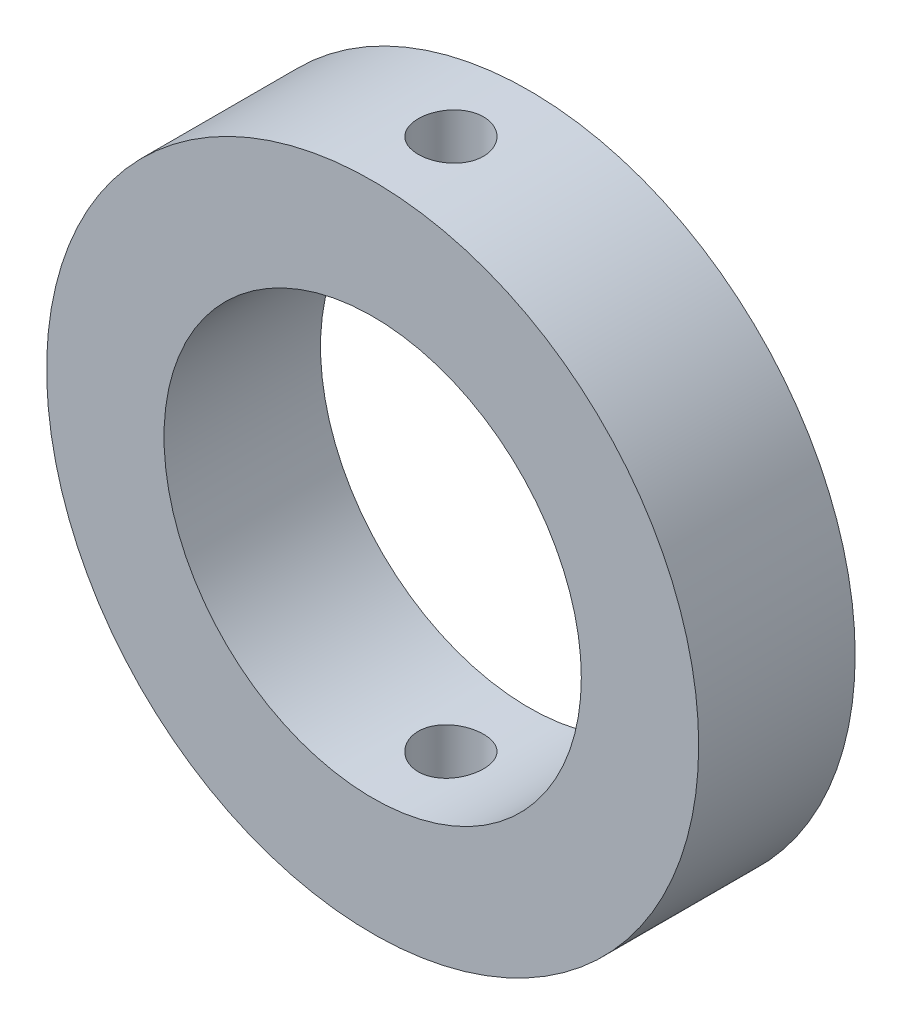
ISO-10303-21;
HEADER;
FILE_DESCRIPTION(('STEP AP214'),'2;1');
FILE_NAME('part.step','',(''),(''),'','','');
FILE_SCHEMA(('AUTOMOTIVE_DESIGN { 1 0 10303 214 1 1 1 1 }'));
ENDSEC;
DATA;
#1=APPLICATION_CONTEXT('core data for automotive mechanical design processes');
#2=APPLICATION_PROTOCOL_DEFINITION('international standard','automotive_design',2000,#1);
#3=PRODUCT_CONTEXT('',#1,'mechanical');
#4=PRODUCT('Part','Part','',(#3));
#5=PRODUCT_RELATED_PRODUCT_CATEGORY('part','',(#4));
#6=PRODUCT_DEFINITION_FORMATION('','',#4);
#7=PRODUCT_DEFINITION_CONTEXT('part definition',#1,'design');
#8=PRODUCT_DEFINITION('design','',#6,#7);
#9=PRODUCT_DEFINITION_SHAPE('','',#8);
#10=(LENGTH_UNIT() NAMED_UNIT(*) SI_UNIT(.MILLI.,.METRE.));
#11=(NAMED_UNIT(*) PLANE_ANGLE_UNIT() SI_UNIT($,.RADIAN.));
#12=(NAMED_UNIT(*) SI_UNIT($,.STERADIAN.) SOLID_ANGLE_UNIT());
#13=UNCERTAINTY_MEASURE_WITH_UNIT(LENGTH_MEASURE(1.E-05),#10,'distance_accuracy_value','');
#14=(GEOMETRIC_REPRESENTATION_CONTEXT(3) GLOBAL_UNCERTAINTY_ASSIGNED_CONTEXT((#13)) GLOBAL_UNIT_ASSIGNED_CONTEXT((#10,
#11,#12)) REPRESENTATION_CONTEXT('',''));
#15=CARTESIAN_POINT('',(0.,0.,0.));
#16=DIRECTION('',(0.,0.,1.));
#17=DIRECTION('',(1.,0.,0.));
#18=AXIS2_PLACEMENT_3D('',#15,#16,#17);
#19=CARTESIAN_POINT('',(0.,0.,12.));
#20=DIRECTION('',(0.,0.,1.));
#21=DIRECTION('',(1.,0.,0.));
#22=AXIS2_PLACEMENT_3D('',#19,#20,#21);
#23=PLANE('',#22);
#24=CARTESIAN_POINT('',(0.,0.,12.));
#25=DIRECTION('',(0.,0.,1.));
#26=DIRECTION('',(1.,0.,0.));
#27=AXIS2_PLACEMENT_3D('',#24,#25,#26);
#28=CIRCLE('',#27,25.);
#29=CARTESIAN_POINT('',(25.,0.,12.));
#30=VERTEX_POINT('',#29);
#31=EDGE_CURVE('E10',#30,#30,#28,.T.);
#32=ORIENTED_EDGE('',*,*,#31,.T.);
#33=EDGE_LOOP('',(#32));
#34=FACE_BOUND('',#33,.T.);
#35=CARTESIAN_POINT('',(0.,0.,12.));
#36=DIRECTION('',(0.,0.,1.));
#37=DIRECTION('',(1.,0.,0.));
#38=AXIS2_PLACEMENT_3D('',#35,#36,#37);
#39=CIRCLE('',#38,16.);
#40=CARTESIAN_POINT('',(16.,0.,12.));
#41=VERTEX_POINT('',#40);
#42=EDGE_CURVE('E57',#41,#41,#39,.T.);
#43=ORIENTED_EDGE('',*,*,#42,.F.);
#44=EDGE_LOOP('',(#43));
#45=FACE_BOUND('',#44,.T.);
#46=ADVANCED_FACE('F40',(#34,#45),#23,.T.);
#47=CARTESIAN_POINT('',(0.,0.,0.));
#48=DIRECTION('',(0.,0.,1.));
#49=DIRECTION('',(1.,0.,0.));
#50=AXIS2_PLACEMENT_3D('',#47,#48,#49);
#51=PLANE('',#50);
#52=CARTESIAN_POINT('',(0.,0.,0.));
#53=DIRECTION('',(0.,0.,1.));
#54=DIRECTION('',(1.,0.,0.));
#55=AXIS2_PLACEMENT_3D('',#52,#53,#54);
#56=CIRCLE('',#55,25.);
#57=CARTESIAN_POINT('',(25.,0.,0.));
#58=VERTEX_POINT('',#57);
#59=EDGE_CURVE('E51',#58,#58,#56,.T.);
#60=ORIENTED_EDGE('',*,*,#59,.F.);
#61=EDGE_LOOP('',(#60));
#62=FACE_BOUND('',#61,.T.);
#63=CARTESIAN_POINT('',(0.,0.,0.));
#64=DIRECTION('',(0.,0.,1.));
#65=DIRECTION('',(1.,0.,0.));
#66=AXIS2_PLACEMENT_3D('',#63,#64,#65);
#67=CIRCLE('',#66,16.);
#68=CARTESIAN_POINT('',(16.,0.,0.));
#69=VERTEX_POINT('',#68);
#70=EDGE_CURVE('E56',#69,#69,#67,.T.);
#71=ORIENTED_EDGE('',*,*,#70,.T.);
#72=EDGE_LOOP('',(#71));
#73=FACE_BOUND('',#72,.T.);
#74=ADVANCED_FACE('F92',(#62,#73),#51,.F.);
#75=CARTESIAN_POINT('',(0.,0.,12.));
#76=DIRECTION('',(0.,0.,-1.));
#77=DIRECTION('',(-1.,0.,0.));
#78=AXIS2_PLACEMENT_3D('',#75,#76,#77);
#79=CYLINDRICAL_SURFACE('',#78,25.);
#80=CARTESIAN_POINT('',(0.,-25.,8.5));
#81=CARTESIAN_POINT('',(0.140050884478893,-24.9999983880192,8.49999393524905));
#82=CARTESIAN_POINT('',(0.280194362919433,-24.9988106399051,8.48819182775889));
#83=CARTESIAN_POINT('',(0.556595996242092,-24.9941866898684,8.44128907427393));
#84=CARTESIAN_POINT('',(0.69284969792207,-24.9907480108506,8.40616275993853));
#85=CARTESIAN_POINT('',(0.957429188633536,-24.9820103640768,8.31364439850542));
#86=CARTESIAN_POINT('',(1.08575971153727,-24.9767125200177,8.25626579870382));
#87=CARTESIAN_POINT('',(1.33094040240102,-24.9648489348577,8.12089773017089));
#88=CARTESIAN_POINT('',(1.44779284694769,-24.9582834459533,8.04291235999965));
#89=CARTESIAN_POINT('',(1.66714887668521,-24.9445936085331,7.86824325584432));
#90=CARTESIAN_POINT('',(1.76960536208723,-24.9374675393466,7.77150050149492));
#91=CARTESIAN_POINT('',(1.95685630357746,-24.9234739226566,7.56218866434242));
#92=CARTESIAN_POINT('',(2.04164994270663,-24.9166063871229,7.44961884989403));
#93=CARTESIAN_POINT('',(2.19133492610904,-24.9038897888196,7.21155367079095));
#94=CARTESIAN_POINT('',(2.2561836636372,-24.8980429177726,7.08603138976285));
#95=CARTESIAN_POINT('',(2.3638659618569,-24.8880509386631,6.82581103523755));
#96=CARTESIAN_POINT('',(2.40670006647823,-24.8839057885556,6.69111318854013));
#97=CARTESIAN_POINT('',(2.46899760400473,-24.8778021018244,6.41684549783498));
#98=CARTESIAN_POINT('',(2.48853913250949,-24.8758362599524,6.27729355786948));
#99=CARTESIAN_POINT('',(2.5039382128384,-24.8742910765131,5.99687784151055));
#100=CARTESIAN_POINT('',(2.499796387177,-24.8747116722186,5.85601409969485));
#101=CARTESIAN_POINT('',(2.4680107006317,-24.8778851724734,5.5775117257667));
#102=CARTESIAN_POINT('',(2.44045211031138,-24.8806296147663,5.43986325167826));
#103=CARTESIAN_POINT('',(2.36274786037647,-24.8881283571855,5.17115509199726));
#104=CARTESIAN_POINT('',(2.31260189563937,-24.8928826844623,5.04009549543742));
#105=CARTESIAN_POINT('',(2.19105223470377,-24.9038752363018,4.78801603175278));
#106=CARTESIAN_POINT('',(2.11961070679995,-24.9101160977039,4.66701452627671));
#107=CARTESIAN_POINT('',(1.95752506838307,-24.923376293322,4.43868696272029));
#108=CARTESIAN_POINT('',(1.86688039584126,-24.9303956503196,4.33136130504559));
#109=CARTESIAN_POINT('',(1.66848528103017,-24.9444596328247,4.13293651502743));
#110=CARTESIAN_POINT('',(1.56066119712841,-24.9515042333249,4.04191099529799));
#111=CARTESIAN_POINT('',(1.33122370434278,-24.964795726963,3.87924091772403));
#112=CARTESIAN_POINT('',(1.209610279999,-24.9710426192064,3.80759638160881));
#113=CARTESIAN_POINT('',(0.955995264230911,-24.9820368916774,3.68572494922437));
#114=CARTESIAN_POINT('',(0.823991865974758,-24.9867840103692,3.63550178795485));
#115=CARTESIAN_POINT('',(0.55336804332483,-24.9942411860352,3.55795270822062));
#116=CARTESIAN_POINT('',(0.414747816941501,-24.9969513039266,3.53062610502344));
#117=CARTESIAN_POINT('',(0.135462747729759,-25.0000212917078,3.49973923066309));
#118=CARTESIAN_POINT('',(-0.00519075526372992,-25.0003912066934,3.49607737936875));
#119=CARTESIAN_POINT('',(-0.285109483289249,-24.9987660439199,3.51235715762191));
#120=CARTESIAN_POINT('',(-0.424374727051175,-24.9967709981117,3.5322984682882));
#121=CARTESIAN_POINT('',(-0.697270517086687,-24.9906465384799,3.59513423855394));
#122=CARTESIAN_POINT('',(-0.830912122430048,-24.986521547951,3.63798113619503));
#123=CARTESIAN_POINT('',(-1.08911080345945,-24.9765999715152,3.74536293509318));
#124=CARTESIAN_POINT('',(-1.21366767539279,-24.9708033481313,3.80989832259849));
#125=CARTESIAN_POINT('',(-1.45062045043036,-24.9581618832606,3.95907709665978));
#126=CARTESIAN_POINT('',(-1.56297414937229,-24.951313590086,4.04378722231454));
#127=CARTESIAN_POINT('',(-1.7719040582797,-24.937348321738,4.23081516935232));
#128=CARTESIAN_POINT('',(-1.86847987212294,-24.9302313398243,4.33313343267579));
#129=CARTESIAN_POINT('',(-2.04346527471786,-24.9165006035189,4.5529164366475));
#130=CARTESIAN_POINT('',(-2.12180819669886,-24.9098887534744,4.67043439135655));
#131=CARTESIAN_POINT('',(-2.25764564685957,-24.8979458115222,4.91701840036671));
#132=CARTESIAN_POINT('',(-2.31514046013471,-24.8926147021009,5.04608429672099));
#133=CARTESIAN_POINT('',(-2.40753802171119,-24.8838486908512,5.31187184866449));
#134=CARTESIAN_POINT('',(-2.44248043702965,-24.8804104612447,5.4485796002278));
#135=CARTESIAN_POINT('',(-2.48891001782366,-24.8758091320719,5.72595799490193));
#136=CARTESIAN_POINT('',(-2.50039785599879,-24.8746459672547,5.86662852423918));
#137=CARTESIAN_POINT('',(-2.49958284617814,-24.8747278276891,6.14727672089176));
#138=CARTESIAN_POINT('',(-2.48738472398278,-24.8759622521752,6.28725470720704));
#139=CARTESIAN_POINT('',(-2.43976363240913,-24.8806775972386,6.56316229292072));
#140=CARTESIAN_POINT('',(-2.4043406369054,-24.884158520343,6.69909188776495));
#141=CARTESIAN_POINT('',(-2.31130421574376,-24.8929717065797,6.96304337261964));
#142=CARTESIAN_POINT('',(-2.25369386085229,-24.898303713509,7.09106635407431));
#143=CARTESIAN_POINT('',(-2.11792888727761,-24.910218795984,7.33564222917759));
#144=CARTESIAN_POINT('',(-2.03977438363854,-24.9168018645238,7.45219518705157));
#145=CARTESIAN_POINT('',(-1.86474639071333,-24.9305121802424,7.67105918617984));
#146=CARTESIAN_POINT('',(-1.76779487222567,-24.9376416181688,7.77330769091772));
#147=CARTESIAN_POINT('',(-1.55807924806277,-24.9516213682196,7.96013058174914));
#148=CARTESIAN_POINT('',(-1.44531136027064,-24.9584716130744,8.04470072839292));
#149=CARTESIAN_POINT('',(-1.20685358540322,-24.971139051729,8.19393363463655));
#150=CARTESIAN_POINT('',(-1.08113187336691,-24.9769536006703,8.25854572736296));
#151=CARTESIAN_POINT('',(-0.820645697751378,-24.9868657312474,8.36565605705967));
#152=CARTESIAN_POINT('',(-0.685891624564024,-24.9909652477413,8.40817922738387));
#153=CARTESIAN_POINT('',(-0.458645653514261,-24.9959553443433,8.45930154271201));
#154=CARTESIAN_POINT('',(-0.367606382111272,-24.9974650172958,8.47454261074839));
#155=CARTESIAN_POINT('',(-0.184391452043282,-24.9994878737697,8.4948938151544));
#156=CARTESIAN_POINT('',(-0.0922157980663944,-25.0000010614006,8.50000399330465));
#157=CARTESIAN_POINT('',(0.,-25.,8.5));
#158=B_SPLINE_CURVE_WITH_KNOTS('',3,(#80,#81,#82,#83,#84,#85,#86,#87,#88,#89,#90,#91,#92,#93,
#94,#95,#96,#97,#98,#99,#100,#101,#102,#103,#104,#105,#106,#107,#108,#109,#110,#111,#112,#113,
#114,#115,#116,#117,#118,#119,#120,#121,#122,#123,#124,#125,#126,#127,#128,#129,#130,#131,#132,
#133,#134,#135,#136,#137,#138,#139,#140,#141,#142,#143,#144,#145,#146,#147,#148,#149,#150,#151,
#152,#153,#154,#155,#156,#157),.UNSPECIFIED.,.T.,.F.,(4,2,2,2,2,2,2,2,2,2,2,2,2,2,2,2,2,2,2,2,2,
2,2,2,2,2,2,2,2,2,2,2,2,2,2,2,2,2,4),(0.,0.419815915671184,0.840094607088716,1.26011971433051,
1.68006134395696,2.10134642155736,2.52265098051765,2.94484938680555,3.3670373610626,
3.78780580112992,4.20856318139441,4.62779493602776,5.04703235404084,5.46701903432237,
5.88701800827813,6.30886835490516,6.73071917449429,7.15264351733954,7.57455524188599,
7.99465471519394,8.41474851297859,8.83397338235762,9.25320765123667,9.67384851871746,
10.0944999452557,10.516666090215,10.9388264618844,11.3602422648251,11.7816459809896,
12.2011907323489,12.620735955651,13.04022313407,13.459707963474,13.8809729356913,
14.3023388159239,14.7247657756561,15.1467148698824,15.4231416808087,15.6995673517257),.UNSPECIFIED.);
#159=CARTESIAN_POINT('',(0.,-25.,8.5));
#160=VERTEX_POINT('',#159);
#161=EDGE_CURVE('E84',#160,#160,#158,.T.);
#162=ORIENTED_EDGE('',*,*,#161,.T.);
#163=EDGE_LOOP('',(#162));
#164=FACE_BOUND('',#163,.T.);
#165=CARTESIAN_POINT('',(0.,25.,8.5));
#166=CARTESIAN_POINT('',(-0.140050884478893,24.9999983880192,8.49999393524905));
#167=CARTESIAN_POINT('',(-0.280194362919433,24.9988106399051,8.48819182775889));
#168=CARTESIAN_POINT('',(-0.556595996242092,24.9941866898684,8.44128907427393));
#169=CARTESIAN_POINT('',(-0.69284969792207,24.9907480108506,8.40616275993853));
#170=CARTESIAN_POINT('',(-0.957429188633536,24.9820103640768,8.31364439850542));
#171=CARTESIAN_POINT('',(-1.08575971153727,24.9767125200177,8.25626579870382));
#172=CARTESIAN_POINT('',(-1.33094040240102,24.9648489348577,8.12089773017089));
#173=CARTESIAN_POINT('',(-1.44779284694769,24.9582834459533,8.04291235999965));
#174=CARTESIAN_POINT('',(-1.66714887668521,24.9445936085331,7.86824325584432));
#175=CARTESIAN_POINT('',(-1.76960536208723,24.9374675393466,7.77150050149492));
#176=CARTESIAN_POINT('',(-1.95685630357746,24.9234739226566,7.56218866434242));
#177=CARTESIAN_POINT('',(-2.04164994270663,24.9166063871229,7.44961884989403));
#178=CARTESIAN_POINT('',(-2.19133492610904,24.9038897888196,7.21155367079095));
#179=CARTESIAN_POINT('',(-2.2561836636372,24.8980429177726,7.08603138976285));
#180=CARTESIAN_POINT('',(-2.3638659618569,24.8880509386631,6.82581103523755));
#181=CARTESIAN_POINT('',(-2.40670006647823,24.8839057885556,6.69111318854013));
#182=CARTESIAN_POINT('',(-2.46899760400473,24.8778021018244,6.41684549783498));
#183=CARTESIAN_POINT('',(-2.48853913250949,24.8758362599524,6.27729355786948));
#184=CARTESIAN_POINT('',(-2.5039382128384,24.8742910765131,5.99687784151055));
#185=CARTESIAN_POINT('',(-2.499796387177,24.8747116722186,5.85601409969485));
#186=CARTESIAN_POINT('',(-2.4680107006317,24.8778851724734,5.5775117257667));
#187=CARTESIAN_POINT('',(-2.44045211031138,24.8806296147663,5.43986325167826));
#188=CARTESIAN_POINT('',(-2.36274786037647,24.8881283571855,5.17115509199726));
#189=CARTESIAN_POINT('',(-2.31260189563937,24.8928826844623,5.04009549543742));
#190=CARTESIAN_POINT('',(-2.19105223470377,24.9038752363018,4.78801603175278));
#191=CARTESIAN_POINT('',(-2.11961070679995,24.9101160977039,4.66701452627671));
#192=CARTESIAN_POINT('',(-1.95752506838307,24.923376293322,4.43868696272029));
#193=CARTESIAN_POINT('',(-1.86688039584126,24.9303956503196,4.33136130504559));
#194=CARTESIAN_POINT('',(-1.66848528103017,24.9444596328247,4.13293651502743));
#195=CARTESIAN_POINT('',(-1.56066119712841,24.9515042333249,4.04191099529799));
#196=CARTESIAN_POINT('',(-1.33122370434278,24.964795726963,3.87924091772403));
#197=CARTESIAN_POINT('',(-1.209610279999,24.9710426192064,3.80759638160881));
#198=CARTESIAN_POINT('',(-0.955995264230911,24.9820368916774,3.68572494922437));
#199=CARTESIAN_POINT('',(-0.823991865974758,24.9867840103692,3.63550178795485));
#200=CARTESIAN_POINT('',(-0.55336804332483,24.9942411860352,3.55795270822062));
#201=CARTESIAN_POINT('',(-0.414747816941501,24.9969513039266,3.53062610502344));
#202=CARTESIAN_POINT('',(-0.135462747729759,25.0000212917078,3.49973923066309));
#203=CARTESIAN_POINT('',(0.00519075526372992,25.0003912066934,3.49607737936875));
#204=CARTESIAN_POINT('',(0.285109483289249,24.9987660439199,3.51235715762191));
#205=CARTESIAN_POINT('',(0.424374727051175,24.9967709981117,3.5322984682882));
#206=CARTESIAN_POINT('',(0.697270517086687,24.9906465384799,3.59513423855394));
#207=CARTESIAN_POINT('',(0.830912122430048,24.986521547951,3.63798113619503));
#208=CARTESIAN_POINT('',(1.08911080345945,24.9765999715152,3.74536293509318));
#209=CARTESIAN_POINT('',(1.21366767539279,24.9708033481313,3.80989832259849));
#210=CARTESIAN_POINT('',(1.45062045043036,24.9581618832606,3.95907709665978));
#211=CARTESIAN_POINT('',(1.56297414937229,24.951313590086,4.04378722231454));
#212=CARTESIAN_POINT('',(1.7719040582797,24.937348321738,4.23081516935232));
#213=CARTESIAN_POINT('',(1.86847987212294,24.9302313398243,4.33313343267579));
#214=CARTESIAN_POINT('',(2.04346527471786,24.9165006035189,4.5529164366475));
#215=CARTESIAN_POINT('',(2.12180819669886,24.9098887534744,4.67043439135655));
#216=CARTESIAN_POINT('',(2.25764564685957,24.8979458115222,4.91701840036671));
#217=CARTESIAN_POINT('',(2.31514046013471,24.8926147021009,5.04608429672099));
#218=CARTESIAN_POINT('',(2.40753802171119,24.8838486908512,5.31187184866449));
#219=CARTESIAN_POINT('',(2.44248043702965,24.8804104612447,5.4485796002278));
#220=CARTESIAN_POINT('',(2.48891001782366,24.8758091320719,5.72595799490193));
#221=CARTESIAN_POINT('',(2.50039785599879,24.8746459672547,5.86662852423918));
#222=CARTESIAN_POINT('',(2.49958284617814,24.8747278276891,6.14727672089176));
#223=CARTESIAN_POINT('',(2.48738472398278,24.8759622521752,6.28725470720704));
#224=CARTESIAN_POINT('',(2.43976363240913,24.8806775972386,6.56316229292072));
#225=CARTESIAN_POINT('',(2.4043406369054,24.884158520343,6.69909188776495));
#226=CARTESIAN_POINT('',(2.31130421574376,24.8929717065797,6.96304337261964));
#227=CARTESIAN_POINT('',(2.25369386085229,24.898303713509,7.09106635407431));
#228=CARTESIAN_POINT('',(2.11792888727761,24.910218795984,7.33564222917759));
#229=CARTESIAN_POINT('',(2.03977438363854,24.9168018645238,7.45219518705157));
#230=CARTESIAN_POINT('',(1.86474639071333,24.9305121802424,7.67105918617984));
#231=CARTESIAN_POINT('',(1.76779487222567,24.9376416181688,7.77330769091772));
#232=CARTESIAN_POINT('',(1.55807924806277,24.9516213682196,7.96013058174914));
#233=CARTESIAN_POINT('',(1.44531136027064,24.9584716130744,8.04470072839292));
#234=CARTESIAN_POINT('',(1.20685358540322,24.971139051729,8.19393363463655));
#235=CARTESIAN_POINT('',(1.08113187336691,24.9769536006703,8.25854572736296));
#236=CARTESIAN_POINT('',(0.820645697751378,24.9868657312474,8.36565605705967));
#237=CARTESIAN_POINT('',(0.685891624564024,24.9909652477413,8.40817922738387));
#238=CARTESIAN_POINT('',(0.458645653514261,24.9959553443433,8.45930154271201));
#239=CARTESIAN_POINT('',(0.367606382111272,24.9974650172958,8.47454261074839));
#240=CARTESIAN_POINT('',(0.184391452043282,24.9994878737697,8.4948938151544));
#241=CARTESIAN_POINT('',(0.0922157980663944,25.0000010614006,8.50000399330465));
#242=CARTESIAN_POINT('',(0.,25.,8.5));
#243=B_SPLINE_CURVE_WITH_KNOTS('',3,(#165,#166,#167,#168,#169,#170,#171,#172,#173,#174,#175,
#176,#177,#178,#179,#180,#181,#182,#183,#184,#185,#186,#187,#188,#189,#190,#191,#192,#193,#194,
#195,#196,#197,#198,#199,#200,#201,#202,#203,#204,#205,#206,#207,#208,#209,#210,#211,#212,#213,
#214,#215,#216,#217,#218,#219,#220,#221,#222,#223,#224,#225,#226,#227,#228,#229,#230,#231,#232,
#233,#234,#235,#236,#237,#238,#239,#240,#241,#242),.UNSPECIFIED.,.T.,.F.,(4,2,2,2,2,2,2,2,2,2,2,
2,2,2,2,2,2,2,2,2,2,2,2,2,2,2,2,2,2,2,2,2,2,2,2,2,2,2,4),(0.,0.419815915671184,
0.840094607088716,1.26011971433051,1.68006134395696,2.10134642155736,2.52265098051765,
2.94484938680555,3.3670373610626,3.78780580112992,4.20856318139441,4.62779493602776,
5.04703235404084,5.46701903432237,5.88701800827813,6.30886835490516,6.73071917449429,
7.15264351733954,7.57455524188599,7.99465471519394,8.41474851297859,8.83397338235762,
9.25320765123667,9.67384851871746,10.0944999452557,10.516666090215,10.9388264618844,
11.3602422648251,11.7816459809896,12.2011907323489,12.620735955651,13.04022313407,
13.459707963474,13.8809729356913,14.3023388159239,14.7247657756561,15.1467148698824,
15.4231416808087,15.6995673517257),.UNSPECIFIED.);
#244=CARTESIAN_POINT('',(0.,25.,8.5));
#245=VERTEX_POINT('',#244);
#246=EDGE_CURVE('E76',#245,#245,#243,.T.);
#247=ORIENTED_EDGE('',*,*,#246,.T.);
#248=EDGE_LOOP('',(#247));
#249=FACE_BOUND('',#248,.T.);
#250=ORIENTED_EDGE('',*,*,#31,.F.);
#251=EDGE_LOOP('',(#250));
#252=FACE_BOUND('',#251,.T.);
#253=ORIENTED_EDGE('',*,*,#59,.T.);
#254=EDGE_LOOP('',(#253));
#255=FACE_BOUND('',#254,.T.);
#256=ADVANCED_FACE('F39',(#164,#249,#252,#255),#79,.T.);
#257=CARTESIAN_POINT('',(0.,0.,12.));
#258=DIRECTION('',(0.,0.,-1.));
#259=DIRECTION('',(-1.,0.,0.));
#260=AXIS2_PLACEMENT_3D('',#257,#258,#259);
#261=CYLINDRICAL_SURFACE('',#260,16.);
#262=CARTESIAN_POINT('',(0.,-16.,8.5));
#263=CARTESIAN_POINT('',(0.139515097271033,-15.9999977019448,8.49999430172848));
#264=CARTESIAN_POINT('',(0.279109404865704,-15.9981561248574,8.48828188622645));
#265=CARTESIAN_POINT('',(0.554391314978102,-15.9909869809759,8.44175630872325));
#266=CARTESIAN_POINT('',(0.690075061323317,-15.9856560884472,8.40692110749649));
#267=CARTESIAN_POINT('',(0.953512538047404,-15.9721069716578,8.31522033719338));
#268=CARTESIAN_POINT('',(1.0812723522899,-15.9638909956317,8.2583719186384));
#269=CARTESIAN_POINT('',(1.3254212510446,-15.9454779403815,8.12430145485839));
#270=CARTESIAN_POINT('',(1.44181181036831,-15.9352811186255,8.04708205696406));
#271=CARTESIAN_POINT('',(1.66091991165162,-15.9139426841436,7.87376695164604));
#272=CARTESIAN_POINT('',(1.76352747914264,-15.9027945139234,7.77753300510975));
#273=CARTESIAN_POINT('',(1.95120768822823,-15.8808607613029,7.56921805173111));
#274=CARTESIAN_POINT('',(2.03627928654192,-15.8700752005075,7.4571361026998));
#275=CARTESIAN_POINT('',(2.18690544328884,-15.8500242812745,7.21956172865627));
#276=CARTESIAN_POINT('',(2.25235273557992,-15.840767397861,7.09400051763821));
#277=CARTESIAN_POINT('',(2.36118681597065,-15.8249120174236,6.8334985891422));
#278=CARTESIAN_POINT('',(2.40457491010063,-15.8183133630222,6.69855842748944));
#279=CARTESIAN_POINT('',(2.46771559322167,-15.8085863451104,6.42428909885621));
#280=CARTESIAN_POINT('',(2.48765705487496,-15.8054302653236,6.2850044141812));
#281=CARTESIAN_POINT('',(2.50392369757622,-15.8028617107177,6.00503281110736));
#282=CARTESIAN_POINT('',(2.50025034860466,-15.8034490028802,5.86434598053396));
#283=CARTESIAN_POINT('',(2.4695458080889,-15.8082755045521,5.58690296814732));
#284=CARTESIAN_POINT('',(2.44272562959693,-15.8124817218495,5.45012277664685));
#285=CARTESIAN_POINT('',(2.36681937833752,-15.8240205634547,5.18302799364068));
#286=CARTESIAN_POINT('',(2.31773262684132,-15.8313532830641,5.05271359935946));
#287=CARTESIAN_POINT('',(2.19846916949384,-15.8483550685462,4.80161128732284));
#288=CARTESIAN_POINT('',(2.12820372315549,-15.8580339308724,4.68086620822693));
#289=CARTESIAN_POINT('',(1.96864058146637,-15.878630461501,4.45280046431446));
#290=CARTESIAN_POINT('',(1.87934153253017,-15.8895482178821,4.34548075511253));
#291=CARTESIAN_POINT('',(1.68309088822333,-15.911537862489,4.14608975336669));
#292=CARTESIAN_POINT('',(1.57595800560539,-15.9226101363559,4.05419684173054));
#293=CARTESIAN_POINT('',(1.34769694737936,-15.9435512534783,3.8896668543601));
#294=CARTESIAN_POINT('',(1.22656870068132,-15.9534200906202,3.81702987644317));
#295=CARTESIAN_POINT('',(0.973595927056491,-15.9708539902704,3.69306192657761));
#296=CARTESIAN_POINT('',(0.84174418624046,-15.9784174854193,3.641745441467));
#297=CARTESIAN_POINT('',(0.571149534696759,-15.9903756000068,3.56203403255277));
#298=CARTESIAN_POINT('',(0.4324071306872,-15.9947704520898,3.53363742593352));
#299=CARTESIAN_POINT('',(0.153508336763735,-15.9998651172728,3.50081072354981));
#300=CARTESIAN_POINT('',(0.0133814615087022,-16.0006027179286,3.49613552102382));
#301=CARTESIAN_POINT('',(-0.265654546411642,-15.9984028649127,3.51023270533598));
#302=CARTESIAN_POINT('',(-0.404563719925156,-15.9954655349964,3.52900430258911));
#303=CARTESIAN_POINT('',(-0.676473446265704,-15.9862692369322,3.58925838768018));
#304=CARTESIAN_POINT('',(-0.809501262056041,-15.9800278421539,3.63062075826773));
#305=CARTESIAN_POINT('',(-1.06673406785663,-15.9649207568356,3.73475509439879));
#306=CARTESIAN_POINT('',(-1.19093861303941,-15.9560549341007,3.79752813844267));
#307=CARTESIAN_POINT('',(-1.42807220225041,-15.9365897274094,3.94327199112658));
#308=CARTESIAN_POINT('',(-1.54090512378373,-15.9259772866342,4.02639742009048));
#309=CARTESIAN_POINT('',(-1.75110696507806,-15.9042388046444,4.21027208590779));
#310=CARTESIAN_POINT('',(-1.84847490447018,-15.8931127309268,4.31102243920485));
#311=CARTESIAN_POINT('',(-2.02588080776691,-15.8714802753665,4.52838119721721));
#312=CARTESIAN_POINT('',(-2.10575398584126,-15.860980411908,4.64512484712233));
#313=CARTESIAN_POINT('',(-2.2447556772664,-15.8419069280583,4.89051607366133));
#314=CARTESIAN_POINT('',(-2.30388478778105,-15.83333325222,5.01916330748948));
#315=CARTESIAN_POINT('',(-2.39946771944995,-15.8191307135236,5.28422964071419));
#316=CARTESIAN_POINT('',(-2.43600654947912,-15.8134908234896,5.42061746876562));
#317=CARTESIAN_POINT('',(-2.48564122040535,-15.8057657028079,5.69768914366398));
#318=CARTESIAN_POINT('',(-2.49873883084997,-15.8036802038444,5.83837266541901));
#319=CARTESIAN_POINT('',(-2.50107452690756,-15.8033105804488,6.11839871590748));
#320=CARTESIAN_POINT('',(-2.49057180548425,-15.804985160429,6.2577390969335));
#321=CARTESIAN_POINT('',(-2.44656223255901,-15.8118569894183,6.53264529714429));
#322=CARTESIAN_POINT('',(-2.41305543086961,-15.8170542307995,6.66821112450172));
#323=CARTESIAN_POINT('',(-2.32408329891852,-15.8303708885491,6.93163782664052));
#324=CARTESIAN_POINT('',(-2.26863761738581,-15.8384876895341,7.05950547825841));
#325=CARTESIAN_POINT('',(-2.13738768546417,-15.856731840474,7.30416561367627));
#326=CARTESIAN_POINT('',(-2.06158262820886,-15.8668592701083,7.42095765828843));
#327=CARTESIAN_POINT('',(-1.8908300813908,-15.8881156809226,7.64146554412683));
#328=CARTESIAN_POINT('',(-1.79569107094768,-15.8992540116029,7.74503219661384));
#329=CARTESIAN_POINT('',(-1.58937594638204,-15.9212004364073,7.93482123638673));
#330=CARTESIAN_POINT('',(-1.47819612078432,-15.9320084534012,8.02103959859188));
#331=CARTESIAN_POINT('',(-1.24216685884341,-15.952151024567,8.17415122303156));
#332=CARTESIAN_POINT('',(-1.11723937214238,-15.9614763443027,8.24092537275961));
#333=CARTESIAN_POINT('',(-0.857851882357782,-15.9775125983888,8.35244099619295));
#334=CARTESIAN_POINT('',(-0.723401776581761,-15.9842262014212,8.39720497255839));
#335=CARTESIAN_POINT('',(-0.490314239911593,-15.9927744586488,8.45343302109059));
#336=CARTESIAN_POINT('',(-0.393105575651623,-15.9954699162612,8.470868490629));
#337=CARTESIAN_POINT('',(-0.197277797850581,-15.9990834869762,8.49415391337908));
#338=CARTESIAN_POINT('',(-0.0986587041691182,-16.0000016250796,8.50000402955734));
#339=CARTESIAN_POINT('',(0.,-16.,8.5));
#340=B_SPLINE_CURVE_WITH_KNOTS('',3,(#262,#263,#264,#265,#266,#267,#268,#269,#270,#271,#272,
#273,#274,#275,#276,#277,#278,#279,#280,#281,#282,#283,#284,#285,#286,#287,#288,#289,#290,#291,
#292,#293,#294,#295,#296,#297,#298,#299,#300,#301,#302,#303,#304,#305,#306,#307,#308,#309,#310,
#311,#312,#313,#314,#315,#316,#317,#318,#319,#320,#321,#322,#323,#324,#325,#326,#327,#328,#329,
#330,#331,#332,#333,#334,#335,#336,#337,#338,#339),.UNSPECIFIED.,.T.,.F.,(4,2,2,2,2,2,2,2,2,2,2,
2,2,2,2,2,2,2,2,2,2,2,2,2,2,2,2,2,2,2,2,2,2,2,2,2,2,2,4),(0.,0.41818474047749,0.836768642528014,
1.25502707944103,1.6732311879203,2.09459568152199,2.51598523645422,2.93963778605759,
3.36326525009238,3.78345631134995,4.20362121670545,4.6199957602258,5.0363829965105,
5.45453977402347,5.87272629892068,6.29545732334367,6.71819049513827,7.14121043754565,
7.56419931829866,7.98280854005914,8.40140366528356,8.81779444756567,9.23420620742031,
9.65388541469672,10.0735912160142,10.4970948024959,10.9205861964898,11.3424741039513,
11.764330162293,12.1815758159869,12.598820566189,13.0156924696662,13.4325808967135,
13.8538201231554,14.275156971423,14.6990230419984,15.1224548565628,15.4181801635154,
15.7139013105871),.UNSPECIFIED.);
#341=CARTESIAN_POINT('',(0.,-16.,8.5));
#342=VERTEX_POINT('',#341);
#343=EDGE_CURVE('E45',#342,#342,#340,.T.);
#344=ORIENTED_EDGE('',*,*,#343,.F.);
#345=EDGE_LOOP('',(#344));
#346=FACE_BOUND('',#345,.T.);
#347=CARTESIAN_POINT('',(0.,16.,8.5));
#348=CARTESIAN_POINT('',(-0.139515097271033,15.9999977019448,8.49999430172848));
#349=CARTESIAN_POINT('',(-0.279109404865704,15.9981561248574,8.48828188622645));
#350=CARTESIAN_POINT('',(-0.554391314978102,15.9909869809759,8.44175630872325));
#351=CARTESIAN_POINT('',(-0.690075061323317,15.9856560884472,8.40692110749649));
#352=CARTESIAN_POINT('',(-0.953512538047404,15.9721069716578,8.31522033719338));
#353=CARTESIAN_POINT('',(-1.0812723522899,15.9638909956317,8.2583719186384));
#354=CARTESIAN_POINT('',(-1.3254212510446,15.9454779403815,8.12430145485839));
#355=CARTESIAN_POINT('',(-1.44181181036831,15.9352811186255,8.04708205696406));
#356=CARTESIAN_POINT('',(-1.66091991165162,15.9139426841436,7.87376695164604));
#357=CARTESIAN_POINT('',(-1.76352747914264,15.9027945139234,7.77753300510975));
#358=CARTESIAN_POINT('',(-1.95120768822823,15.8808607613029,7.56921805173111));
#359=CARTESIAN_POINT('',(-2.03627928654192,15.8700752005075,7.4571361026998));
#360=CARTESIAN_POINT('',(-2.18690544328884,15.8500242812745,7.21956172865627));
#361=CARTESIAN_POINT('',(-2.25235273557992,15.840767397861,7.09400051763821));
#362=CARTESIAN_POINT('',(-2.36118681597065,15.8249120174236,6.8334985891422));
#363=CARTESIAN_POINT('',(-2.40457491010063,15.8183133630222,6.69855842748944));
#364=CARTESIAN_POINT('',(-2.46771559322167,15.8085863451104,6.42428909885621));
#365=CARTESIAN_POINT('',(-2.48765705487496,15.8054302653236,6.2850044141812));
#366=CARTESIAN_POINT('',(-2.50392369757622,15.8028617107177,6.00503281110736));
#367=CARTESIAN_POINT('',(-2.50025034860466,15.8034490028802,5.86434598053396));
#368=CARTESIAN_POINT('',(-2.4695458080889,15.8082755045521,5.58690296814732));
#369=CARTESIAN_POINT('',(-2.44272562959693,15.8124817218495,5.45012277664685));
#370=CARTESIAN_POINT('',(-2.36681937833752,15.8240205634547,5.18302799364068));
#371=CARTESIAN_POINT('',(-2.31773262684132,15.8313532830641,5.05271359935946));
#372=CARTESIAN_POINT('',(-2.19846916949384,15.8483550685462,4.80161128732284));
#373=CARTESIAN_POINT('',(-2.12820372315549,15.8580339308724,4.68086620822693));
#374=CARTESIAN_POINT('',(-1.96864058146637,15.878630461501,4.45280046431446));
#375=CARTESIAN_POINT('',(-1.87934153253017,15.8895482178821,4.34548075511253));
#376=CARTESIAN_POINT('',(-1.68309088822333,15.911537862489,4.14608975336669));
#377=CARTESIAN_POINT('',(-1.57595800560539,15.9226101363559,4.05419684173054));
#378=CARTESIAN_POINT('',(-1.34769694737936,15.9435512534783,3.8896668543601));
#379=CARTESIAN_POINT('',(-1.22656870068132,15.9534200906202,3.81702987644317));
#380=CARTESIAN_POINT('',(-0.973595927056491,15.9708539902704,3.69306192657761));
#381=CARTESIAN_POINT('',(-0.84174418624046,15.9784174854193,3.641745441467));
#382=CARTESIAN_POINT('',(-0.571149534696759,15.9903756000068,3.56203403255277));
#383=CARTESIAN_POINT('',(-0.4324071306872,15.9947704520898,3.53363742593352));
#384=CARTESIAN_POINT('',(-0.153508336763735,15.9998651172728,3.50081072354981));
#385=CARTESIAN_POINT('',(-0.0133814615087022,16.0006027179286,3.49613552102382));
#386=CARTESIAN_POINT('',(0.265654546411642,15.9984028649127,3.51023270533598));
#387=CARTESIAN_POINT('',(0.404563719925156,15.9954655349964,3.52900430258911));
#388=CARTESIAN_POINT('',(0.676473446265704,15.9862692369322,3.58925838768018));
#389=CARTESIAN_POINT('',(0.809501262056041,15.9800278421539,3.63062075826773));
#390=CARTESIAN_POINT('',(1.06673406785663,15.9649207568356,3.73475509439879));
#391=CARTESIAN_POINT('',(1.19093861303941,15.9560549341007,3.79752813844267));
#392=CARTESIAN_POINT('',(1.42807220225041,15.9365897274094,3.94327199112658));
#393=CARTESIAN_POINT('',(1.54090512378373,15.9259772866342,4.02639742009048));
#394=CARTESIAN_POINT('',(1.75110696507806,15.9042388046444,4.21027208590779));
#395=CARTESIAN_POINT('',(1.84847490447018,15.8931127309268,4.31102243920485));
#396=CARTESIAN_POINT('',(2.02588080776691,15.8714802753665,4.52838119721721));
#397=CARTESIAN_POINT('',(2.10575398584126,15.860980411908,4.64512484712233));
#398=CARTESIAN_POINT('',(2.2447556772664,15.8419069280583,4.89051607366133));
#399=CARTESIAN_POINT('',(2.30388478778105,15.83333325222,5.01916330748948));
#400=CARTESIAN_POINT('',(2.39946771944995,15.8191307135236,5.28422964071419));
#401=CARTESIAN_POINT('',(2.43600654947912,15.8134908234896,5.42061746876562));
#402=CARTESIAN_POINT('',(2.48564122040535,15.8057657028079,5.69768914366398));
#403=CARTESIAN_POINT('',(2.49873883084997,15.8036802038444,5.83837266541901));
#404=CARTESIAN_POINT('',(2.50107452690756,15.8033105804488,6.11839871590748));
#405=CARTESIAN_POINT('',(2.49057180548425,15.804985160429,6.2577390969335));
#406=CARTESIAN_POINT('',(2.44656223255901,15.8118569894183,6.53264529714429));
#407=CARTESIAN_POINT('',(2.41305543086961,15.8170542307995,6.66821112450172));
#408=CARTESIAN_POINT('',(2.32408329891852,15.8303708885491,6.93163782664052));
#409=CARTESIAN_POINT('',(2.26863761738581,15.8384876895341,7.05950547825841));
#410=CARTESIAN_POINT('',(2.13738768546417,15.856731840474,7.30416561367627));
#411=CARTESIAN_POINT('',(2.06158262820886,15.8668592701083,7.42095765828843));
#412=CARTESIAN_POINT('',(1.8908300813908,15.8881156809226,7.64146554412683));
#413=CARTESIAN_POINT('',(1.79569107094768,15.8992540116029,7.74503219661384));
#414=CARTESIAN_POINT('',(1.58937594638204,15.9212004364073,7.93482123638673));
#415=CARTESIAN_POINT('',(1.47819612078432,15.9320084534012,8.02103959859188));
#416=CARTESIAN_POINT('',(1.24216685884341,15.952151024567,8.17415122303156));
#417=CARTESIAN_POINT('',(1.11723937214238,15.9614763443027,8.24092537275961));
#418=CARTESIAN_POINT('',(0.857851882357782,15.9775125983888,8.35244099619295));
#419=CARTESIAN_POINT('',(0.723401776581761,15.9842262014212,8.39720497255839));
#420=CARTESIAN_POINT('',(0.490314239911593,15.9927744586488,8.45343302109059));
#421=CARTESIAN_POINT('',(0.393105575651623,15.9954699162612,8.470868490629));
#422=CARTESIAN_POINT('',(0.197277797850581,15.9990834869762,8.49415391337908));
#423=CARTESIAN_POINT('',(0.0986587041691182,16.0000016250796,8.50000402955734));
#424=CARTESIAN_POINT('',(0.,16.,8.5));
#425=B_SPLINE_CURVE_WITH_KNOTS('',3,(#347,#348,#349,#350,#351,#352,#353,#354,#355,#356,#357,
#358,#359,#360,#361,#362,#363,#364,#365,#366,#367,#368,#369,#370,#371,#372,#373,#374,#375,#376,
#377,#378,#379,#380,#381,#382,#383,#384,#385,#386,#387,#388,#389,#390,#391,#392,#393,#394,#395,
#396,#397,#398,#399,#400,#401,#402,#403,#404,#405,#406,#407,#408,#409,#410,#411,#412,#413,#414,
#415,#416,#417,#418,#419,#420,#421,#422,#423,#424),.UNSPECIFIED.,.T.,.F.,(4,2,2,2,2,2,2,2,2,2,2,
2,2,2,2,2,2,2,2,2,2,2,2,2,2,2,2,2,2,2,2,2,2,2,2,2,2,2,4),(0.,0.41818474047749,0.836768642528014,
1.25502707944103,1.6732311879203,2.09459568152199,2.51598523645422,2.93963778605759,
3.36326525009238,3.78345631134995,4.20362121670545,4.6199957602258,5.0363829965105,
5.45453977402347,5.87272629892068,6.29545732334367,6.71819049513827,7.14121043754565,
7.56419931829866,7.98280854005914,8.40140366528356,8.81779444756567,9.23420620742031,
9.65388541469672,10.0735912160142,10.4970948024959,10.9205861964898,11.3424741039513,
11.764330162293,12.1815758159869,12.598820566189,13.0156924696662,13.4325808967135,
13.8538201231554,14.275156971423,14.6990230419984,15.1224548565628,15.4181801635154,
15.7139013105871),.UNSPECIFIED.);
#426=CARTESIAN_POINT('',(0.,16.,8.5));
#427=VERTEX_POINT('',#426);
#428=EDGE_CURVE('E62',#427,#427,#425,.T.);
#429=ORIENTED_EDGE('',*,*,#428,.F.);
#430=EDGE_LOOP('',(#429));
#431=FACE_BOUND('',#430,.T.);
#432=ORIENTED_EDGE('',*,*,#42,.T.);
#433=EDGE_LOOP('',(#432));
#434=FACE_BOUND('',#433,.T.);
#435=ORIENTED_EDGE('',*,*,#70,.F.);
#436=EDGE_LOOP('',(#435));
#437=FACE_BOUND('',#436,.T.);
#438=ADVANCED_FACE('F67',(#346,#431,#434,#437),#261,.F.);
#439=CARTESIAN_POINT('',(0.,-40.,6.));
#440=DIRECTION('',(0.,1.,0.));
#441=DIRECTION('',(0.,0.,1.));
#442=AXIS2_PLACEMENT_3D('',#439,#440,#441);
#443=CYLINDRICAL_SURFACE('',#442,2.5);
#444=ORIENTED_EDGE('',*,*,#428,.T.);
#445=EDGE_LOOP('',(#444));
#446=FACE_BOUND('',#445,.T.);
#447=ORIENTED_EDGE('',*,*,#246,.F.);
#448=EDGE_LOOP('',(#447));
#449=FACE_BOUND('',#448,.T.);
#450=ADVANCED_FACE('F75',(#446,#449),#443,.F.);
#451=ORIENTED_EDGE('',*,*,#343,.T.);
#452=EDGE_LOOP('',(#451));
#453=FACE_BOUND('',#452,.T.);
#454=ORIENTED_EDGE('',*,*,#161,.F.);
#455=EDGE_LOOP('',(#454));
#456=FACE_BOUND('',#455,.T.);
#457=ADVANCED_FACE('F69',(#453,#456),#443,.F.);
#458=CLOSED_SHELL('',(#46,#74,#256,#438,#450,#457));
#459=MANIFOLD_SOLID_BREP('B2',#458);
#460=ADVANCED_BREP_SHAPE_REPRESENTATION('',(#18,#459),#14);
#461=SHAPE_DEFINITION_REPRESENTATION(#9,#460);
ENDSEC;
END-ISO-10303-21;
